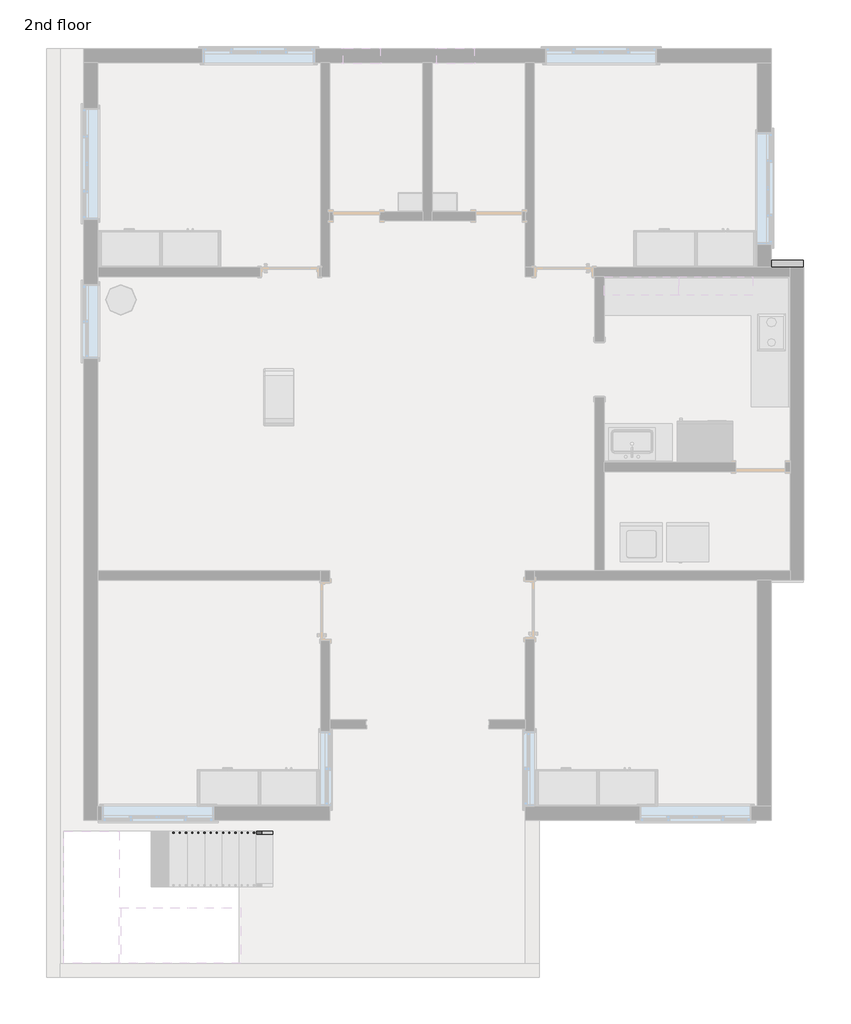
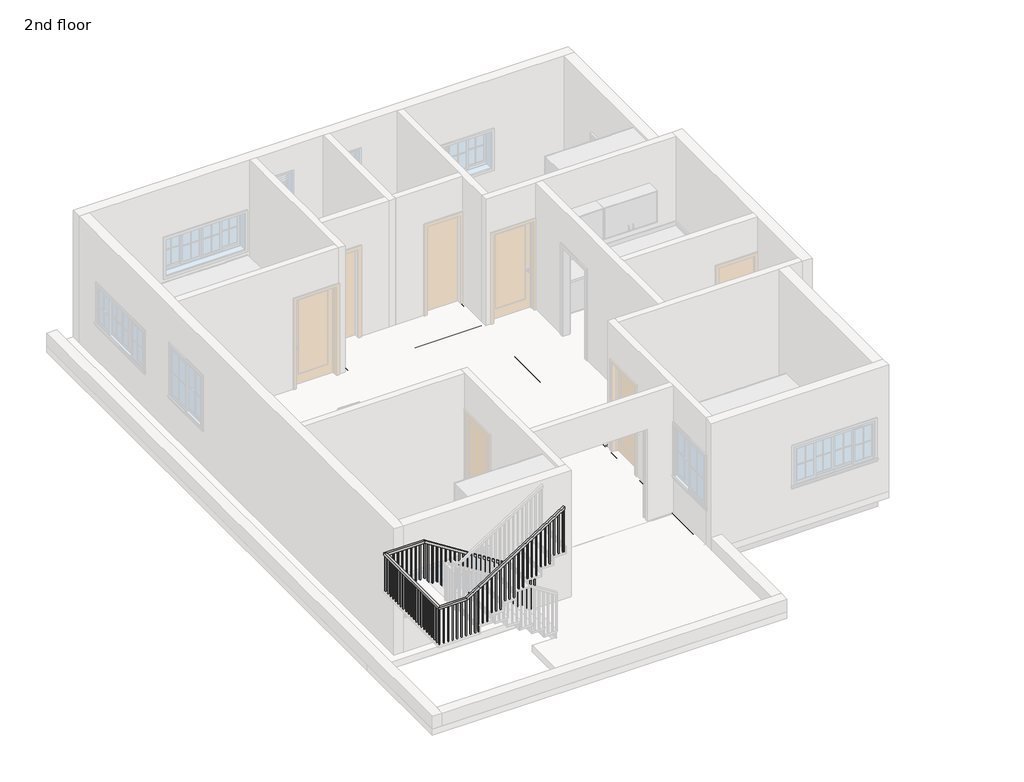
# One storey, part 2 of 4: 6 beams, 1 railing.
"""IFC4 building model written with IfcOpenShell, lengths in millimetres."""

from ifc_helpers import new_model, si_unit, frame, origin, place, context, project, spatial, polyline, outline, extrude, faceted_brep, element, save

model = new_model("IFC4")

# Units and contexts
model_context = context("Model", 3, world=origin())
ifc_project = project(units=[si_unit("LENGTHUNIT", "METRE", prefix="MILLI")], contexts=[model_context])

# Site, building, storey
site = spatial("IfcSite", under=ifc_project)
building = spatial("IfcBuilding", under=site)
storey = spatial("IfcBuildingStorey", under=building, Name="2nd floor", Elevation=7010.4)

# Beams
placement = place(None, origin())
element("IfcBeam", 1, ObjectType="Concrete-Rectangular Beam", at=placement, inside=storey, context=model_context, shape_type="Brep", body=[
    faceted_brep([(-12413.6124084, 10142.6961804, 7010.4), (-12413.6124084, 9914.0961804, 7010.4), (-8794.1124084, 9914.0961804, 7010.4), (-8565.5124084, 9914.0961804, 7010.4), (-7117.7124084, 9914.0961804, 7010.4), (-6889.1124084, 9914.0961804, 7010.4), (-5441.3124084, 9914.0961804, 7010.4), (-5212.7124084, 9914.0961804, 7010.4), (-1593.2124084, 9914.0961804, 7010.4), (-1593.2124084, 10142.6961804, 7010.4), (-5174.6124084, 10142.6961804, 7010.4), (-5174.6124084, 9952.1961804, 7010.4), (-5479.4124084, 9952.1961804, 7010.4), (-5479.4124084, 10142.6961804, 7010.4), (-8451.2124084, 10142.6961804, 7010.4), (-8451.2124084, 9952.1961804, 7010.4), (-8756.0124084, 9952.1961804, 7010.4), (-8756.0124084, 10142.6961804, 7010.4), (-12413.6124084, 9914.0961804, 6705.6), (-8794.1124084, 9914.0961804, 6705.6), (-8565.5124084, 9914.0961804, 6705.6), (-7117.7124084, 9914.0961804, 6705.6), (-6889.1124084, 9914.0961804, 6705.6), (-5441.3124084, 9914.0961804, 6705.6), (-5212.7124084, 9914.0961804, 6705.6), (-1593.2124084, 9914.0961804, 6705.6), (-12413.6124084, 10142.6961804, 6705.6), (-8756.0124084, 10142.6961804, 6705.6), (-8756.0124084, 9952.1961804, 6705.6), (-8451.2124084, 9952.1961804, 6705.6), (-8451.2124084, 10142.6961804, 6705.6), (-5479.4124084, 10142.6961804, 6705.6), (-5479.4124084, 9952.1961804, 6705.6), (-5174.6124084, 9952.1961804, 6705.6), (-5174.6124084, 10142.6961804, 6705.6), (-1593.2124084, 10142.6961804, 6705.6)], [[[0, 1, 2, 3, 4, 5, 6, 7, 8, 9, 10, 11, 12, 13, 14, 15, 16, 17]], [[1, 18, 19, 20, 21, 22, 23, 24, 25, 8, 7, 6, 5, 4, 3, 2]], [[18, 26, 27, 28, 29, 30, 31, 32, 33, 34, 35, 25, 24, 23, 22, 21, 20, 19]], [[26, 0, 17, 27]], [[1, 0, 26, 18]], [[9, 8, 25, 35]], [[29, 15, 14, 30]], [[15, 29, 28, 16]], [[16, 28, 27, 17]], [[9, 35, 34, 10]], [[33, 11, 10, 34]], [[11, 33, 32, 12]], [[12, 32, 31, 13]], [[30, 14, 13, 31]]]),
])
element("IfcBeam", 2, ObjectType="Concrete-Rectangular Beam", at=placement, inside=storey, context=model_context, shape_type="SweptSolid", body=[
    extrude(outline(polyline([(-1593.2124084, 9875.9961804), (-1364.6124084, 9875.9961804), (-1364.6124084, 6751.7961804), (-1593.2124084, 6751.7961804), (-1593.2124084, 9875.9961804)])), frame((0.0, 0.0, 6705.6), z_axis=(0.0, 0.0, 1.0), x_axis=(1.0, 0.0, 0.0)), (0.0, 0.0, 1.0), 304.8),
])
element("IfcBeam", 3, ObjectType="Concrete-Rectangular Beam", at=placement, inside=storey, context=model_context, shape_type="Brep", body=[
    faceted_brep([(-843.9124084, 6713.6961804, 7010.4), (-843.9124084, 6485.0961804, 7010.4), (-843.9124084, 6485.0961804, 6705.6), (-843.9124084, 6713.6961804, 6705.6), (-1364.6124084, 6713.6961804, 7010.4), (-1364.6124084, 6485.0961804, 7010.4), (-1364.6124084, 6485.0961804, 6705.6), (-1364.6124084, 6713.6961804, 6705.6)], [[[0, 1, 2, 3]], [[1, 0, 4, 5]], [[2, 1, 5, 6]], [[3, 2, 6, 7]], [[0, 3, 7, 4]], [[5, 4, 7, 6]]]),
    faceted_brep([(-12413.6124084, 6485.0961804, 7010.4), (-12413.6124084, 6713.6961804, 7010.4), (-12413.6124084, 6713.6961804, 6705.6), (-12413.6124084, 6485.0961804, 6705.6), (-8756.0124084, 6713.6961804, 7010.4), (-8756.0124084, 6485.0961804, 7010.4), (-8756.0124084, 6485.0961804, 6705.6), (-8756.0124084, 6713.6961804, 6705.6), (-8794.1124084, 6485.0961804, 7010.4), (-8794.1124084, 6713.6961804, 7010.4), (-8794.1124084, 6485.0961804, 6705.6), (-8794.1124084, 6713.6961804, 6705.6)], [[[0, 1, 2, 3]], [[4, 5, 6, 7]], [[1, 0, 8, 5, 4, 9]], [[0, 3, 10, 6, 5, 8]], [[3, 2, 11, 7, 6, 10]], [[2, 1, 9, 4, 7, 11]]]),
    faceted_brep([(-1593.2124084, 6713.6961804, 7010.4), (-1593.2124084, 6485.0961804, 7010.4), (-1593.2124084, 6485.0961804, 6705.6), (-1593.2124084, 6713.6961804, 6705.6), (-5212.7124084, 6713.6961804, 7010.4), (-5250.8124084, 6713.6961804, 7010.4), (-5250.8124084, 6485.0961804, 7010.4), (-5212.7124084, 6485.0961804, 7010.4), (-5250.8124084, 6485.0961804, 6705.6), (-5212.7124084, 6485.0961804, 6705.6), (-5250.8124084, 6713.6961804, 6705.6), (-5212.7124084, 6713.6961804, 6705.6)], [[[0, 1, 2, 3]], [[1, 0, 4, 5, 6, 7]], [[2, 1, 7, 6, 8, 9]], [[3, 2, 9, 8, 10, 11]], [[0, 3, 11, 10, 5, 4]], [[6, 5, 10, 8]]]),
    faceted_brep([(-8527.4124084, 6485.0961804, 7010.4), (-8527.4124084, 6713.6961804, 7010.4), (-8527.4124084, 6713.6961804, 6705.6), (-8527.4124084, 6485.0961804, 6705.6), (-5479.4124084, 6713.6961804, 7010.4), (-5479.4124084, 6485.0961804, 7010.4), (-5479.4124084, 6485.0961804, 6705.6), (-5479.4124084, 6713.6961804, 6705.6)], [[[0, 1, 2, 3]], [[4, 5, 6, 7]], [[1, 0, 5, 4]], [[0, 3, 6, 5]], [[3, 2, 7, 6]], [[2, 1, 4, 7]]]),
])
element("IfcBeam", 4, ObjectType="Concrete-Rectangular Beam", at=placement, inside=storey, context=model_context, shape_type="Brep", body=[
    faceted_brep([(-5212.7124084, 9914.0961804, 7010.4), (-5441.3124084, 9914.0961804, 7010.4), (-5441.3124084, 7551.8961804, 7010.4), (-5441.3124084, 7323.2961804, 7010.4), (-5441.3124084, 6751.7961804, 7010.4), (-5250.8124084, 6751.7961804, 7010.4), (-5250.8124084, 6713.6961804, 7010.4), (-5212.7124084, 6713.6961804, 7010.4), (-5212.7124084, 9914.0961804, 6705.6), (-5212.7124084, 6713.6961804, 6705.6), (-5441.3124084, 9914.0961804, 6705.6), (-5250.8124084, 6713.6961804, 6705.6), (-5250.8124084, 6751.7961804, 6705.6), (-5441.3124084, 6751.7961804, 6705.6), (-5441.3124084, 7323.2961804, 6705.6), (-5441.3124084, 7551.8961804, 6705.6)], [[[0, 1, 2, 3, 4, 5, 6, 7]], [[8, 0, 7, 9]], [[10, 8, 9, 11, 12, 13, 14, 15]], [[1, 10, 15, 14, 13, 4, 3, 2]], [[1, 0, 8, 10]], [[9, 7, 6, 11]], [[12, 5, 4, 13]], [[5, 12, 11, 6]]]),
    faceted_brep([(-5212.7124084, -2201.7038196, 7010.4), (-5441.3124084, -2201.7038196, 7010.4), (-5441.3124084, -2201.7038196, 6705.6), (-5212.7124084, -2201.7038196, 6705.6), (-5441.3124084, 1430.4961804, 6705.6), (-5441.3124084, 1430.4961804, 7010.4), (-5212.7124084, 1430.4961804, 7010.4), (-5212.7124084, 1430.4961804, 6705.6), (-5441.3124084, -779.3038196, 6705.6), (-5441.3124084, -1007.9038196, 6705.6), (-5441.3124084, -1007.9038196, 7010.4), (-5441.3124084, -779.3038196, 7010.4)], [[[0, 1, 2, 3]], [[4, 5, 6, 7]], [[5, 4, 8, 9, 2, 1, 10, 11]], [[1, 0, 6, 5, 11, 10]], [[0, 3, 7, 6]], [[3, 2, 9, 8, 4, 7]]]),
    faceted_brep([(-5212.7124084, 6485.0961804, 7010.4), (-5212.7124084, 6485.0961804, 6705.6), (-5250.8124084, 6485.0961804, 6705.6), (-5250.8124084, 6485.0961804, 7010.4), (-5250.8124084, 6446.9961804, 7010.4), (-5441.3124084, 6446.9961804, 7010.4), (-5441.3124084, 1659.0961804, 7010.4), (-5403.2124084, 1659.0961804, 7010.4), (-5403.2124084, 1697.1961804, 7010.4), (-5212.7124084, 1697.1961804, 7010.4), (-5212.7124084, 1697.1961804, 6705.6), (-5403.2124084, 1697.1961804, 6705.6), (-5403.2124084, 1659.0961804, 6705.6), (-5441.3124084, 1659.0961804, 6705.6), (-5441.3124084, 6446.9961804, 6705.6), (-5250.8124084, 6446.9961804, 6705.6)], [[[0, 1, 2, 3]], [[0, 3, 4, 5, 6, 7, 8, 9]], [[1, 0, 9, 10]], [[2, 1, 10, 11, 12, 13, 14, 15]], [[6, 13, 12, 7]], [[13, 6, 5, 14]], [[15, 4, 3, 2]], [[4, 15, 14, 5]], [[8, 11, 10, 9]], [[11, 8, 7, 12]]]),
])
element("IfcBeam", 5, ObjectType="Concrete-Rectangular Beam", at=placement, inside=storey, context=model_context, shape_type="SweptSolid", body=[
    extrude(outline(polyline([(-7117.7124084, 9914.0961804), (-6889.1124084, 9914.0961804), (-6889.1124084, 7551.8961804), (-7117.7124084, 7551.8961804), (-7117.7124084, 9914.0961804)])), frame((0.0, 0.0, 6705.6), z_axis=(0.0, 0.0, 1.0), x_axis=(1.0, 0.0, 0.0)), (0.0, 0.0, 1.0), 304.8),
])
element("IfcBeam", 6, ObjectType="Concrete-Rectangular Beam", at=placement, inside=storey, context=model_context, shape_type="Brep", body=[
    faceted_brep([(-5441.3124084, 7323.2961804, 7010.4), (-5441.3124084, 7551.8961804, 7010.4), (-6889.1124084, 7551.8961804, 7010.4), (-7117.7124084, 7551.8961804, 7010.4), (-8565.5124084, 7551.8961804, 7010.4), (-8565.5124084, 7323.2961804, 7010.4), (-5441.3124084, 7323.2961804, 6705.6), (-8565.5124084, 7323.2961804, 6705.6), (-5441.3124084, 7551.8961804, 6705.6), (-8565.5124084, 7551.8961804, 6705.6), (-7117.7124084, 7551.8961804, 6705.6), (-6889.1124084, 7551.8961804, 6705.6)], [[[0, 1, 2, 3, 4, 5]], [[6, 0, 5, 7]], [[8, 6, 7, 9, 10, 11]], [[1, 8, 11, 10, 9, 4, 3, 2]], [[1, 0, 6, 8]], [[5, 4, 9, 7]]]),
])

# Railing
element("IfcRailing", 7, ObjectType="Handrail - Rectangular", at=placement, inside=storey, context=model_context, shape_type="SolidModel", body=[
    faceted_brep([(-9543.8120641, -2698.7669819, 8102.6), (-9543.8120641, -2698.7669819, 8042.386276), (-9543.8120641, -2647.9669819, 8042.386276), (-9543.8120641, -2647.9669819, 8102.6), (-12058.4120641, -2698.7669819, 9702.8), (-12073.205059, -2698.7669819, 9652.0), (-12073.205059, -2647.9669819, 9652.0), (-12058.4120641, -2647.9669819, 9702.8), (-12922.0120641, -2698.7669819, 9702.8), (-12922.0120641, -2698.7669819, 9652.0), (-12972.8120641, -2647.9669819, 9652.0), (-12972.8120641, -2647.9669819, 9702.8), (-12922.0120641, -4767.1038196, 9702.8), (-12922.0120641, -4767.1038196, 9652.0), (-12972.8120641, -4817.9038196, 9652.0), (-12972.8120641, -4817.9038196, 9702.8), (-12337.8120641, -4767.1038196, 9702.8), (-12323.0190691, -4767.1038196, 9652.0), (-12323.0190691, -4817.9038196, 9652.0), (-12337.8120641, -4817.9038196, 9702.8), (-12058.4120641, -4767.1038196, 9880.6), (-12031.138789, -4767.1038196, 9837.7419964), (-12031.138789, -4817.9038196, 9837.7419964), (-12058.4120641, -4817.9038196, 9880.6), (-10102.6120641, -4767.1038196, 11125.2), (-10102.6120641, -4817.9038196, 11125.2), (-10102.6120641, -4817.9038196, 11064.986276), (-10102.6120641, -4767.1038196, 11064.986276)], [[[0, 1, 2, 3]], [[1, 0, 4, 5]], [[2, 1, 5, 6]], [[3, 2, 6, 7]], [[0, 3, 7, 4]], [[5, 4, 8, 9]], [[6, 5, 9, 10]], [[7, 6, 10, 11]], [[4, 7, 11, 8]], [[9, 8, 12, 13]], [[10, 9, 13, 14]], [[11, 10, 14, 15]], [[8, 11, 15, 12]], [[13, 12, 16, 17]], [[14, 13, 17, 18]], [[15, 14, 18, 19]], [[12, 15, 19, 16]], [[17, 16, 20, 21]], [[18, 17, 21, 22]], [[19, 18, 22, 23]], [[16, 19, 23, 20]], [[24, 25, 26, 27]], [[21, 20, 24, 27]], [[22, 21, 27, 26]], [[23, 22, 26, 25]], [[20, 23, 25, 24]]]),
    extrude(outline(polyline([(11054.8840032, -10118.4870641), (11042.761276, -10137.5370641), (10033.0, -10137.5370641), (10033.0, -10118.4870641), (11054.8840032, -10118.4870641)])), frame((0.0, -4802.0288196, 0.0), z_axis=(0.0, 1.0, 0.0), x_axis=(0.0, 0.0, 1.0)), (0.0, 0.0, 1.0), 19.05),
    extrude(outline(polyline([(10990.2294578, -10220.0870641), (10978.1067305, -10239.1370641), (10033.0, -10239.1370641), (10033.0, -10220.0870641), (10990.2294578, -10220.0870641)])), frame((0.0, -4802.0288196, 0.0), z_axis=(0.0, 1.0, 0.0), x_axis=(0.0, 0.0, 1.0)), (0.0, 0.0, 1.0), 19.05),
    extrude(outline(polyline([(10925.5749123, -10321.6870641), (10913.4521851, -10340.7370641), (10033.0, -10340.7370641), (10033.0, -10321.6870641), (10925.5749123, -10321.6870641)])), frame((0.0, -4802.0288196, 0.0), z_axis=(0.0, 1.0, 0.0), x_axis=(0.0, 0.0, 1.0)), (0.0, 0.0, 1.0), 19.05),
    extrude(outline(polyline([(10860.9203669, -10423.2870641), (10848.7976396, -10442.3370641), (9855.2, -10442.3370641), (9855.2, -10423.2870641), (10860.9203669, -10423.2870641)])), frame((0.0, -4802.0288196, 0.0), z_axis=(0.0, 1.0, 0.0), x_axis=(0.0, 0.0, 1.0)), (0.0, 0.0, 1.0), 19.05),
    extrude(outline(polyline([(10796.2658214, -10524.8870641), (10784.1430941, -10543.9370641), (9855.2, -10543.9370641), (9855.2, -10524.8870641), (10796.2658214, -10524.8870641)])), frame((0.0, -4802.0288196, 0.0), z_axis=(0.0, 1.0, 0.0), x_axis=(0.0, 0.0, 1.0)), (0.0, 0.0, 1.0), 19.05),
    extrude(outline(polyline([(10731.611276, -10626.4870641), (10719.4885487, -10645.5370641), (9855.2, -10645.5370641), (9855.2, -10626.4870641), (10731.611276, -10626.4870641)])), frame((0.0, -4802.0288196, 0.0), z_axis=(0.0, 1.0, 0.0), x_axis=(0.0, 0.0, 1.0)), (0.0, 0.0, 1.0), 19.05),
    extrude(outline(polyline([(10666.9567305, -10728.0870641), (10654.8340032, -10747.1370641), (9677.4, -10747.1370641), (9677.4, -10728.0870641), (10666.9567305, -10728.0870641)])), frame((0.0, -4802.0288196, 0.0), z_axis=(0.0, 1.0, 0.0), x_axis=(0.0, 0.0, 1.0)), (0.0, 0.0, 1.0), 19.05),
    extrude(outline(polyline([(10602.3021851, -10829.6870641), (10590.1794578, -10848.7370641), (9677.4, -10848.7370641), (9677.4, -10829.6870641), (10602.3021851, -10829.6870641)])), frame((0.0, -4802.0288196, 0.0), z_axis=(0.0, 1.0, 0.0), x_axis=(0.0, 0.0, 1.0)), (0.0, 0.0, 1.0), 19.05),
    extrude(outline(polyline([(10537.6476396, -10931.2870641), (10525.5249123, -10950.3370641), (9677.4, -10950.3370641), (9677.4, -10931.2870641), (10537.6476396, -10931.2870641)])), frame((0.0, -4802.0288196, 0.0), z_axis=(0.0, 1.0, 0.0), x_axis=(0.0, 0.0, 1.0)), (0.0, 0.0, 1.0), 19.05),
    extrude(outline(polyline([(10472.9930941, -11032.8870641), (10460.8703669, -11051.9370641), (9499.6, -11051.9370641), (9499.6, -11032.8870641), (10472.9930941, -11032.8870641)])), frame((0.0, -4802.0288196, 0.0), z_axis=(0.0, 1.0, 0.0), x_axis=(0.0, 0.0, 1.0)), (0.0, 0.0, 1.0), 19.05),
    extrude(outline(polyline([(10408.3385487, -11134.4870641), (10396.2158214, -11153.5370641), (9499.6, -11153.5370641), (9499.6, -11134.4870641), (10408.3385487, -11134.4870641)])), frame((0.0, -4802.0288196, 0.0), z_axis=(0.0, 1.0, 0.0), x_axis=(0.0, 0.0, 1.0)), (0.0, 0.0, 1.0), 19.05),
    extrude(outline(polyline([(10343.6840032, -11236.0870641), (10331.561276, -11255.1370641), (9321.8, -11255.1370641), (9321.8, -11236.0870641), (10343.6840032, -11236.0870641)])), frame((0.0, -4802.0288196, 0.0), z_axis=(0.0, 1.0, 0.0), x_axis=(0.0, 0.0, 1.0)), (0.0, 0.0, 1.0), 19.05),
    extrude(outline(polyline([(10279.0294578, -11337.6870641), (10266.9067305, -11356.7370641), (9321.8, -11356.7370641), (9321.8, -11337.6870641), (10279.0294578, -11337.6870641)])), frame((0.0, -4802.0288196, 0.0), z_axis=(0.0, 1.0, 0.0), x_axis=(0.0, 0.0, 1.0)), (0.0, 0.0, 1.0), 19.05),
    extrude(outline(polyline([(10214.3749123, -11439.2870641), (10202.2521851, -11458.3370641), (9321.8, -11458.3370641), (9321.8, -11439.2870641), (10214.3749123, -11439.2870641)])), frame((0.0, -4802.0288196, 0.0), z_axis=(0.0, 1.0, 0.0), x_axis=(0.0, 0.0, 1.0)), (0.0, 0.0, 1.0), 19.05),
    extrude(outline(polyline([(10149.7203669, -11540.8870641), (10137.5976396, -11559.9370641), (9144.0, -11559.9370641), (9144.0, -11540.8870641), (10149.7203669, -11540.8870641)])), frame((0.0, -4802.0288196, 0.0), z_axis=(0.0, 1.0, 0.0), x_axis=(0.0, 0.0, 1.0)), (0.0, 0.0, 1.0), 19.05),
    extrude(outline(polyline([(10085.0658214, -11642.4870641), (10072.9430941, -11661.5370641), (9144.0, -11661.5370641), (9144.0, -11642.4870641), (10085.0658214, -11642.4870641)])), frame((0.0, -4802.0288196, 0.0), z_axis=(0.0, 1.0, 0.0), x_axis=(0.0, 0.0, 1.0)), (0.0, 0.0, 1.0), 19.05),
    extrude(outline(polyline([(10020.411276, -11744.0870641), (10008.2885487, -11763.1370641), (9144.0, -11763.1370641), (9144.0, -11744.0870641), (10020.411276, -11744.0870641)])), frame((0.0, -4802.0288196, 0.0), z_axis=(0.0, 1.0, 0.0), x_axis=(0.0, 0.0, 1.0)), (0.0, 0.0, 1.0), 19.05),
    extrude(outline(polyline([(9955.7567305, -11845.6870641), (9943.6340032, -11864.7370641), (8966.2, -11864.7370641), (8966.2, -11845.6870641), (9955.7567305, -11845.6870641)])), frame((0.0, -4802.0288196, 0.0), z_axis=(0.0, 1.0, 0.0), x_axis=(0.0, 0.0, 1.0)), (0.0, 0.0, 1.0), 19.05),
    extrude(outline(polyline([(9891.1021851, -11947.2870641), (9878.9794578, -11966.3370641), (8966.2, -11966.3370641), (8966.2, -11947.2870641), (9891.1021851, -11947.2870641)])), frame((0.0, -4802.0288196, 0.0), z_axis=(0.0, 1.0, 0.0), x_axis=(0.0, 0.0, 1.0)), (0.0, 0.0, 1.0), 19.05),
    extrude(outline(polyline([(9777.9567305, -12125.0870641), (9765.8340032, -12144.1370641), (8788.4, -12144.1370641), (8788.4, -12125.0870641), (9777.9567305, -12125.0870641)])), frame((0.0, -4802.0288196, 0.0), z_axis=(0.0, 1.0, 0.0), x_axis=(0.0, 0.0, 1.0)), (0.0, 0.0, 1.0), 19.05),
    extrude(outline(polyline([(9713.3021851, -12226.6870641), (9701.1794578, -12245.7370641), (8788.4, -12245.7370641), (8788.4, -12226.6870641), (9713.3021851, -12226.6870641)])), frame((0.0, -4802.0288196, 0.0), z_axis=(0.0, 1.0, 0.0), x_axis=(0.0, 0.0, 1.0)), (0.0, 0.0, 1.0), 19.05),
    extrude(outline(polyline([(-12347.3370641, -4802.0288196), (-12347.3370641, -4782.9788196), (-12328.2870641, -4782.9788196), (-12328.2870641, -4802.0288196), (-12347.3370641, -4802.0288196)])), frame((0.0, 0.0, 8788.4), z_axis=(0.0, 0.0, 1.0), x_axis=(1.0, 0.0, 0.0)), (0.0, 0.0, 1.0), 863.6),
    extrude(outline(polyline([(-12448.9370641, -4802.0288196), (-12448.9370641, -4782.9788196), (-12429.8870641, -4782.9788196), (-12429.8870641, -4802.0288196), (-12448.9370641, -4802.0288196)])), frame((0.0, 0.0, 8788.4), z_axis=(0.0, 0.0, 1.0), x_axis=(1.0, 0.0, 0.0)), (0.0, 0.0, 1.0), 863.6),
    extrude(outline(polyline([(-12550.5370641, -4802.0288196), (-12550.5370641, -4782.9788196), (-12531.4870641, -4782.9788196), (-12531.4870641, -4802.0288196), (-12550.5370641, -4802.0288196)])), frame((0.0, 0.0, 8788.4), z_axis=(0.0, 0.0, 1.0), x_axis=(1.0, 0.0, 0.0)), (0.0, 0.0, 1.0), 863.6),
    extrude(outline(polyline([(-12652.1370641, -4802.0288196), (-12652.1370641, -4782.9788196), (-12633.0870641, -4782.9788196), (-12633.0870641, -4802.0288196), (-12652.1370641, -4802.0288196)])), frame((0.0, 0.0, 8788.4), z_axis=(0.0, 0.0, 1.0), x_axis=(1.0, 0.0, 0.0)), (0.0, 0.0, 1.0), 863.6),
    extrude(outline(polyline([(-12753.7370641, -4802.0288196), (-12753.7370641, -4782.9788196), (-12734.6870641, -4782.9788196), (-12734.6870641, -4802.0288196), (-12753.7370641, -4802.0288196)])), frame((0.0, 0.0, 8788.4), z_axis=(0.0, 0.0, 1.0), x_axis=(1.0, 0.0, 0.0)), (0.0, 0.0, 1.0), 863.6),
    extrude(outline(polyline([(-12855.3370641, -4802.0288196), (-12855.3370641, -4782.9788196), (-12836.2870641, -4782.9788196), (-12836.2870641, -4802.0288196), (-12855.3370641, -4802.0288196)])), frame((0.0, 0.0, 8788.4), z_axis=(0.0, 0.0, 1.0), x_axis=(1.0, 0.0, 0.0)), (0.0, 0.0, 1.0), 863.6),
    extrude(outline(polyline([(-12956.9370641, -4695.8419819), (-12937.8870641, -4695.8419819), (-12937.8870641, -4714.8919819), (-12956.9370641, -4714.8919819), (-12956.9370641, -4695.8419819)])), frame((0.0, 0.0, 8788.4), z_axis=(0.0, 0.0, 1.0), x_axis=(1.0, 0.0, 0.0)), (0.0, 0.0, 1.0), 863.6),
    extrude(outline(polyline([(-12956.9370641, -4594.2419819), (-12937.8870641, -4594.2419819), (-12937.8870641, -4613.2919819), (-12956.9370641, -4613.2919819), (-12956.9370641, -4594.2419819)])), frame((0.0, 0.0, 8788.4), z_axis=(0.0, 0.0, 1.0), x_axis=(1.0, 0.0, 0.0)), (0.0, 0.0, 1.0), 863.6),
    extrude(outline(polyline([(-12956.9370641, -4492.6419819), (-12937.8870641, -4492.6419819), (-12937.8870641, -4511.6919819), (-12956.9370641, -4511.6919819), (-12956.9370641, -4492.6419819)])), frame((0.0, 0.0, 8788.4), z_axis=(0.0, 0.0, 1.0), x_axis=(1.0, 0.0, 0.0)), (0.0, 0.0, 1.0), 863.6),
    extrude(outline(polyline([(-12956.9370641, -4391.0419819), (-12937.8870641, -4391.0419819), (-12937.8870641, -4410.0919819), (-12956.9370641, -4410.0919819), (-12956.9370641, -4391.0419819)])), frame((0.0, 0.0, 8788.4), z_axis=(0.0, 0.0, 1.0), x_axis=(1.0, 0.0, 0.0)), (0.0, 0.0, 1.0), 863.6),
    extrude(outline(polyline([(-12956.9370641, -4289.4419819), (-12937.8870641, -4289.4419819), (-12937.8870641, -4308.4919819), (-12956.9370641, -4308.4919819), (-12956.9370641, -4289.4419819)])), frame((0.0, 0.0, 8788.4), z_axis=(0.0, 0.0, 1.0), x_axis=(1.0, 0.0, 0.0)), (0.0, 0.0, 1.0), 863.6),
    extrude(outline(polyline([(-12956.9370641, -4187.8419819), (-12937.8870641, -4187.8419819), (-12937.8870641, -4206.8919819), (-12956.9370641, -4206.8919819), (-12956.9370641, -4187.8419819)])), frame((0.0, 0.0, 8788.4), z_axis=(0.0, 0.0, 1.0), x_axis=(1.0, 0.0, 0.0)), (0.0, 0.0, 1.0), 863.6),
    extrude(outline(polyline([(-12956.9370641, -4086.2419819), (-12937.8870641, -4086.2419819), (-12937.8870641, -4105.2919819), (-12956.9370641, -4105.2919819), (-12956.9370641, -4086.2419819)])), frame((0.0, 0.0, 8788.4), z_axis=(0.0, 0.0, 1.0), x_axis=(1.0, 0.0, 0.0)), (0.0, 0.0, 1.0), 863.6),
    extrude(outline(polyline([(-12956.9370641, -3984.6419819), (-12937.8870641, -3984.6419819), (-12937.8870641, -4003.6919819), (-12956.9370641, -4003.6919819), (-12956.9370641, -3984.6419819)])), frame((0.0, 0.0, 8788.4), z_axis=(0.0, 0.0, 1.0), x_axis=(1.0, 0.0, 0.0)), (0.0, 0.0, 1.0), 863.6),
    extrude(outline(polyline([(-12956.9370641, -3883.0419819), (-12937.8870641, -3883.0419819), (-12937.8870641, -3902.0919819), (-12956.9370641, -3902.0919819), (-12956.9370641, -3883.0419819)])), frame((0.0, 0.0, 8788.4), z_axis=(0.0, 0.0, 1.0), x_axis=(1.0, 0.0, 0.0)), (0.0, 0.0, 1.0), 863.6),
    extrude(outline(polyline([(-12956.9370641, -3781.4419819), (-12937.8870641, -3781.4419819), (-12937.8870641, -3800.4919819), (-12956.9370641, -3800.4919819), (-12956.9370641, -3781.4419819)])), frame((0.0, 0.0, 8788.4), z_axis=(0.0, 0.0, 1.0), x_axis=(1.0, 0.0, 0.0)), (0.0, 0.0, 1.0), 863.6),
    extrude(outline(polyline([(-12956.9370641, -3679.8419819), (-12937.8870641, -3679.8419819), (-12937.8870641, -3698.8919819), (-12956.9370641, -3698.8919819), (-12956.9370641, -3679.8419819)])), frame((0.0, 0.0, 8788.4), z_axis=(0.0, 0.0, 1.0), x_axis=(1.0, 0.0, 0.0)), (0.0, 0.0, 1.0), 863.6),
    extrude(outline(polyline([(-12956.9370641, -3578.2419819), (-12937.8870641, -3578.2419819), (-12937.8870641, -3597.2919819), (-12956.9370641, -3597.2919819), (-12956.9370641, -3578.2419819)])), frame((0.0, 0.0, 8788.4), z_axis=(0.0, 0.0, 1.0), x_axis=(1.0, 0.0, 0.0)), (0.0, 0.0, 1.0), 863.6),
    extrude(outline(polyline([(-12956.9370641, -3476.6419819), (-12937.8870641, -3476.6419819), (-12937.8870641, -3495.6919819), (-12956.9370641, -3495.6919819), (-12956.9370641, -3476.6419819)])), frame((0.0, 0.0, 8788.4), z_axis=(0.0, 0.0, 1.0), x_axis=(1.0, 0.0, 0.0)), (0.0, 0.0, 1.0), 863.6),
    extrude(outline(polyline([(-12956.9370641, -3375.0419819), (-12937.8870641, -3375.0419819), (-12937.8870641, -3394.0919819), (-12956.9370641, -3394.0919819), (-12956.9370641, -3375.0419819)])), frame((0.0, 0.0, 8788.4), z_axis=(0.0, 0.0, 1.0), x_axis=(1.0, 0.0, 0.0)), (0.0, 0.0, 1.0), 863.6),
    extrude(outline(polyline([(-12956.9370641, -3273.4419819), (-12937.8870641, -3273.4419819), (-12937.8870641, -3292.4919819), (-12956.9370641, -3292.4919819), (-12956.9370641, -3273.4419819)])), frame((0.0, 0.0, 8788.4), z_axis=(0.0, 0.0, 1.0), x_axis=(1.0, 0.0, 0.0)), (0.0, 0.0, 1.0), 863.6),
    extrude(outline(polyline([(-12956.9370641, -3171.8419819), (-12937.8870641, -3171.8419819), (-12937.8870641, -3190.8919819), (-12956.9370641, -3190.8919819), (-12956.9370641, -3171.8419819)])), frame((0.0, 0.0, 8788.4), z_axis=(0.0, 0.0, 1.0), x_axis=(1.0, 0.0, 0.0)), (0.0, 0.0, 1.0), 863.6),
    extrude(outline(polyline([(-12956.9370641, -3070.2419819), (-12937.8870641, -3070.2419819), (-12937.8870641, -3089.2919819), (-12956.9370641, -3089.2919819), (-12956.9370641, -3070.2419819)])), frame((0.0, 0.0, 8788.4), z_axis=(0.0, 0.0, 1.0), x_axis=(1.0, 0.0, 0.0)), (0.0, 0.0, 1.0), 863.6),
    extrude(outline(polyline([(-12956.9370641, -2968.6419819), (-12937.8870641, -2968.6419819), (-12937.8870641, -2987.6919819), (-12956.9370641, -2987.6919819), (-12956.9370641, -2968.6419819)])), frame((0.0, 0.0, 8788.4), z_axis=(0.0, 0.0, 1.0), x_axis=(1.0, 0.0, 0.0)), (0.0, 0.0, 1.0), 863.6),
    extrude(outline(polyline([(-12956.9370641, -2867.0419819), (-12937.8870641, -2867.0419819), (-12937.8870641, -2886.0919819), (-12956.9370641, -2886.0919819), (-12956.9370641, -2867.0419819)])), frame((0.0, 0.0, 8788.4), z_axis=(0.0, 0.0, 1.0), x_axis=(1.0, 0.0, 0.0)), (0.0, 0.0, 1.0), 863.6),
    extrude(outline(polyline([(-12956.9370641, -2765.4419819), (-12937.8870641, -2765.4419819), (-12937.8870641, -2784.4919819), (-12956.9370641, -2784.4919819), (-12956.9370641, -2765.4419819)])), frame((0.0, 0.0, 8788.4), z_axis=(0.0, 0.0, 1.0), x_axis=(1.0, 0.0, 0.0)), (0.0, 0.0, 1.0), 863.6),
    extrude(outline(polyline([(-12861.6870641, -2663.8419819), (-12861.6870641, -2682.8919819), (-12880.7370641, -2682.8919819), (-12880.7370641, -2663.8419819), (-12861.6870641, -2663.8419819)])), frame((0.0, 0.0, 8788.4), z_axis=(0.0, 0.0, 1.0), x_axis=(1.0, 0.0, 0.0)), (0.0, 0.0, 1.0), 863.6),
    extrude(outline(polyline([(-12760.0870641, -2663.8419819), (-12760.0870641, -2682.8919819), (-12779.1370641, -2682.8919819), (-12779.1370641, -2663.8419819), (-12760.0870641, -2663.8419819)])), frame((0.0, 0.0, 8788.4), z_axis=(0.0, 0.0, 1.0), x_axis=(1.0, 0.0, 0.0)), (0.0, 0.0, 1.0), 863.6),
    extrude(outline(polyline([(-12658.4870641, -2663.8419819), (-12658.4870641, -2682.8919819), (-12677.5370641, -2682.8919819), (-12677.5370641, -2663.8419819), (-12658.4870641, -2663.8419819)])), frame((0.0, 0.0, 8788.4), z_axis=(0.0, 0.0, 1.0), x_axis=(1.0, 0.0, 0.0)), (0.0, 0.0, 1.0), 863.6),
    extrude(outline(polyline([(-12556.8870641, -2663.8419819), (-12556.8870641, -2682.8919819), (-12575.9370641, -2682.8919819), (-12575.9370641, -2663.8419819), (-12556.8870641, -2663.8419819)])), frame((0.0, 0.0, 8788.4), z_axis=(0.0, 0.0, 1.0), x_axis=(1.0, 0.0, 0.0)), (0.0, 0.0, 1.0), 863.6),
    extrude(outline(polyline([(-12455.2870641, -2663.8419819), (-12455.2870641, -2682.8919819), (-12474.3370641, -2682.8919819), (-12474.3370641, -2663.8419819), (-12455.2870641, -2663.8419819)])), frame((0.0, 0.0, 8788.4), z_axis=(0.0, 0.0, 1.0), x_axis=(1.0, 0.0, 0.0)), (0.0, 0.0, 1.0), 863.6),
    extrude(outline(polyline([(-12353.6870641, -2663.8419819), (-12353.6870641, -2682.8919819), (-12372.7370641, -2682.8919819), (-12372.7370641, -2663.8419819), (-12353.6870641, -2663.8419819)])), frame((0.0, 0.0, 8788.4), z_axis=(0.0, 0.0, 1.0), x_axis=(1.0, 0.0, 0.0)), (0.0, 0.0, 1.0), 863.6),
    extrude(outline(polyline([(-12252.0870641, -2663.8419819), (-12252.0870641, -2682.8919819), (-12271.1370641, -2682.8919819), (-12271.1370641, -2663.8419819), (-12252.0870641, -2663.8419819)])), frame((0.0, 0.0, 8788.4), z_axis=(0.0, 0.0, 1.0), x_axis=(1.0, 0.0, 0.0)), (0.0, 0.0, 1.0), 863.6),
    extrude(outline(polyline([(-12150.4870641, -2663.8419819), (-12150.4870641, -2682.8919819), (-12169.5370641, -2682.8919819), (-12169.5370641, -2663.8419819), (-12150.4870641, -2663.8419819)])), frame((0.0, 0.0, 8788.4), z_axis=(0.0, 0.0, 1.0), x_axis=(1.0, 0.0, 0.0)), (0.0, 0.0, 1.0), 863.6),
    extrude(outline(polyline([(9588.0340032, -11972.6870641), (9600.1567305, -11991.7370641), (8610.6, -11991.7370641), (8610.6, -11972.6870641), (9588.0340032, -11972.6870641)])), frame((0.0, -2682.8919819, 0.0), z_axis=(0.0, 1.0, 0.0), x_axis=(0.0, 0.0, 1.0)), (0.0, 0.0, 1.0), 19.05),
    extrude(outline(polyline([(9523.3794578, -11871.0870641), (9535.5021851, -11890.1370641), (8610.6, -11890.1370641), (8610.6, -11871.0870641), (9523.3794578, -11871.0870641)])), frame((0.0, -2682.8919819, 0.0), z_axis=(0.0, 1.0, 0.0), x_axis=(0.0, 0.0, 1.0)), (0.0, 0.0, 1.0), 19.05),
    extrude(outline(polyline([(9458.7249123, -11769.4870641), (9470.8476396, -11788.5370641), (8610.6, -11788.5370641), (8610.6, -11769.4870641), (9458.7249123, -11769.4870641)])), frame((0.0, -2682.8919819, 0.0), z_axis=(0.0, 1.0, 0.0), x_axis=(0.0, 0.0, 1.0)), (0.0, 0.0, 1.0), 19.05),
    extrude(outline(polyline([(9394.0703669, -11667.8870641), (9406.1930941, -11686.9370641), (8432.8, -11686.9370641), (8432.8, -11667.8870641), (9394.0703669, -11667.8870641)])), frame((0.0, -2682.8919819, 0.0), z_axis=(0.0, 1.0, 0.0), x_axis=(0.0, 0.0, 1.0)), (0.0, 0.0, 1.0), 19.05),
    extrude(outline(polyline([(9329.4158214, -11566.2870641), (9341.5385487, -11585.3370641), (8432.8, -11585.3370641), (8432.8, -11566.2870641), (9329.4158214, -11566.2870641)])), frame((0.0, -2682.8919819, 0.0), z_axis=(0.0, 1.0, 0.0), x_axis=(0.0, 0.0, 1.0)), (0.0, 0.0, 1.0), 19.05),
    extrude(outline(polyline([(9264.761276, -11464.6870641), (9276.8840032, -11483.7370641), (8255.0, -11483.7370641), (8255.0, -11464.6870641), (9264.761276, -11464.6870641)])), frame((0.0, -2682.8919819, 0.0), z_axis=(0.0, 1.0, 0.0), x_axis=(0.0, 0.0, 1.0)), (0.0, 0.0, 1.0), 19.05),
    extrude(outline(polyline([(9200.1067305, -11363.0870641), (9212.2294578, -11382.1370641), (8255.0, -11382.1370641), (8255.0, -11363.0870641), (9200.1067305, -11363.0870641)])), frame((0.0, -2682.8919819, 0.0), z_axis=(0.0, 1.0, 0.0), x_axis=(0.0, 0.0, 1.0)), (0.0, 0.0, 1.0), 19.05),
    extrude(outline(polyline([(9135.4521851, -11261.4870641), (9147.5749123, -11280.5370641), (8255.0, -11280.5370641), (8255.0, -11261.4870641), (9135.4521851, -11261.4870641)])), frame((0.0, -2682.8919819, 0.0), z_axis=(0.0, 1.0, 0.0), x_axis=(0.0, 0.0, 1.0)), (0.0, 0.0, 1.0), 19.05),
    extrude(outline(polyline([(9070.7976396, -11159.8870641), (9082.9203669, -11178.9370641), (8077.2, -11178.9370641), (8077.2, -11159.8870641), (9070.7976396, -11159.8870641)])), frame((0.0, -2682.8919819, 0.0), z_axis=(0.0, 1.0, 0.0), x_axis=(0.0, 0.0, 1.0)), (0.0, 0.0, 1.0), 19.05),
    extrude(outline(polyline([(9006.1430941, -11058.2870641), (9018.2658214, -11077.3370641), (8077.2, -11077.3370641), (8077.2, -11058.2870641), (9006.1430941, -11058.2870641)])), frame((0.0, -2682.8919819, 0.0), z_axis=(0.0, 1.0, 0.0), x_axis=(0.0, 0.0, 1.0)), (0.0, 0.0, 1.0), 19.05),
    extrude(outline(polyline([(8941.4885487, -10956.6870641), (8953.611276, -10975.7370641), (8077.2, -10975.7370641), (8077.2, -10956.6870641), (8941.4885487, -10956.6870641)])), frame((0.0, -2682.8919819, 0.0), z_axis=(0.0, 1.0, 0.0), x_axis=(0.0, 0.0, 1.0)), (0.0, 0.0, 1.0), 19.05),
    extrude(outline(polyline([(8876.8340032, -10855.0870641), (8888.9567305, -10874.1370641), (7899.4, -10874.1370641), (7899.4, -10855.0870641), (8876.8340032, -10855.0870641)])), frame((0.0, -2682.8919819, 0.0), z_axis=(0.0, 1.0, 0.0), x_axis=(0.0, 0.0, 1.0)), (0.0, 0.0, 1.0), 19.05),
    extrude(outline(polyline([(8812.1794578, -10753.4870641), (8824.3021851, -10772.5370641), (7899.4, -10772.5370641), (7899.4, -10753.4870641), (8812.1794578, -10753.4870641)])), frame((0.0, -2682.8919819, 0.0), z_axis=(0.0, 1.0, 0.0), x_axis=(0.0, 0.0, 1.0)), (0.0, 0.0, 1.0), 19.05),
    extrude(outline(polyline([(8747.5249123, -10651.8870641), (8759.6476396, -10670.9370641), (7899.4, -10670.9370641), (7899.4, -10651.8870641), (8747.5249123, -10651.8870641)])), frame((0.0, -2682.8919819, 0.0), z_axis=(0.0, 1.0, 0.0), x_axis=(0.0, 0.0, 1.0)), (0.0, 0.0, 1.0), 19.05),
    extrude(outline(polyline([(8682.8703669, -10550.2870641), (8694.9930941, -10569.3370641), (7721.6, -10569.3370641), (7721.6, -10550.2870641), (8682.8703669, -10550.2870641)])), frame((0.0, -2682.8919819, 0.0), z_axis=(0.0, 1.0, 0.0), x_axis=(0.0, 0.0, 1.0)), (0.0, 0.0, 1.0), 19.05),
    extrude(outline(polyline([(8618.2158214, -10448.6870641), (8630.3385487, -10467.7370641), (7721.6, -10467.7370641), (7721.6, -10448.6870641), (8618.2158214, -10448.6870641)])), frame((0.0, -2682.8919819, 0.0), z_axis=(0.0, 1.0, 0.0), x_axis=(0.0, 0.0, 1.0)), (0.0, 0.0, 1.0), 19.05),
    extrude(outline(polyline([(8553.561276, -10347.0870641), (8565.6840032, -10366.1370641), (7543.8, -10366.1370641), (7543.8, -10347.0870641), (8553.561276, -10347.0870641)])), frame((0.0, -2682.8919819, 0.0), z_axis=(0.0, 1.0, 0.0), x_axis=(0.0, 0.0, 1.0)), (0.0, 0.0, 1.0), 19.05),
    extrude(outline(polyline([(8488.9067305, -10245.4870641), (8501.0294578, -10264.5370641), (7543.8, -10264.5370641), (7543.8, -10245.4870641), (8488.9067305, -10245.4870641)])), frame((0.0, -2682.8919819, 0.0), z_axis=(0.0, 1.0, 0.0), x_axis=(0.0, 0.0, 1.0)), (0.0, 0.0, 1.0), 19.05),
    extrude(outline(polyline([(8424.2521851, -10143.8870641), (8436.3749123, -10162.9370641), (7543.8, -10162.9370641), (7543.8, -10143.8870641), (8424.2521851, -10143.8870641)])), frame((0.0, -2682.8919819, 0.0), z_axis=(0.0, 1.0, 0.0), x_axis=(0.0, 0.0, 1.0)), (0.0, 0.0, 1.0), 19.05),
    extrude(outline(polyline([(8359.5976396, -10042.2870641), (8371.7203669, -10061.3370641), (7366.0, -10061.3370641), (7366.0, -10042.2870641), (8359.5976396, -10042.2870641)])), frame((0.0, -2682.8919819, 0.0), z_axis=(0.0, 1.0, 0.0), x_axis=(0.0, 0.0, 1.0)), (0.0, 0.0, 1.0), 19.05),
    extrude(outline(polyline([(8294.9430941, -9940.6870641), (8307.0658214, -9959.7370641), (7366.0, -9959.7370641), (7366.0, -9940.6870641), (8294.9430941, -9940.6870641)])), frame((0.0, -2682.8919819, 0.0), z_axis=(0.0, 1.0, 0.0), x_axis=(0.0, 0.0, 1.0)), (0.0, 0.0, 1.0), 19.05),
    extrude(outline(polyline([(8230.2885487, -9839.0870641), (8242.411276, -9858.1370641), (7366.0, -9858.1370641), (7366.0, -9839.0870641), (8230.2885487, -9839.0870641)])), frame((0.0, -2682.8919819, 0.0), z_axis=(0.0, 1.0, 0.0), x_axis=(0.0, 0.0, 1.0)), (0.0, 0.0, 1.0), 19.05),
    extrude(outline(polyline([(8165.6340032, -9737.4870641), (8177.7567305, -9756.5370641), (7188.2, -9756.5370641), (7188.2, -9737.4870641), (8165.6340032, -9737.4870641)])), frame((0.0, -2682.8919819, 0.0), z_axis=(0.0, 1.0, 0.0), x_axis=(0.0, 0.0, 1.0)), (0.0, 0.0, 1.0), 19.05),
    extrude(outline(polyline([(8100.9794578, -9635.8870641), (8113.1021851, -9654.9370641), (7188.2, -9654.9370641), (7188.2, -9635.8870641), (8100.9794578, -9635.8870641)])), frame((0.0, -2682.8919819, 0.0), z_axis=(0.0, 1.0, 0.0), x_axis=(0.0, 0.0, 1.0)), (0.0, 0.0, 1.0), 19.05),
    extrude(outline(polyline([(9826.4476396, -12048.8870641), (9814.3249123, -12067.9370641), (8788.4, -12067.9370641), (8788.4, -12048.8870641), (9826.4476396, -12048.8870641)])), frame((0.0, -4802.0288196, 0.0), z_axis=(0.0, 1.0, 0.0), x_axis=(0.0, 0.0, 1.0)), (0.0, 0.0, 1.0), 19.05),
    extrude(outline(polyline([(-12956.9370641, -4782.9788196), (-12937.8870641, -4782.9788196), (-12937.8870641, -4802.0288196), (-12956.9370641, -4802.0288196), (-12956.9370641, -4782.9788196)])), frame((0.0, 0.0, 8788.4), z_axis=(0.0, 0.0, 1.0), x_axis=(1.0, 0.0, 0.0)), (0.0, 0.0, 1.0), 863.6),
    extrude(outline(polyline([(-12937.8870641, -2663.8419819), (-12937.8870641, -2682.8919819), (-12956.9370641, -2682.8919819), (-12956.9370641, -2663.8419819), (-12937.8870641, -2663.8419819)])), frame((0.0, 0.0, 8788.4), z_axis=(0.0, 0.0, 1.0), x_axis=(1.0, 0.0, 0.0)), (0.0, 0.0, 1.0), 863.6),
    extrude(outline(polyline([(9636.5249123, -12048.8870641), (9648.6476396, -12067.9370641), (8788.4, -12067.9370641), (8788.4, -12048.8870641), (9636.5249123, -12048.8870641)])), frame((0.0, -2682.8919819, 0.0), z_axis=(0.0, 1.0, 0.0), x_axis=(0.0, 0.0, 1.0)), (0.0, 0.0, 1.0), 19.05),
    extrude(outline(polyline([(11064.986276, -10102.6120641), (11052.8635487, -10121.6620641), (10033.0, -10121.6620641), (10033.0, -10102.6120641), (11064.986276, -10102.6120641)])), frame((0.0, -4802.0288196, 0.0), z_axis=(0.0, 1.0, 0.0), x_axis=(0.0, 0.0, 1.0)), (0.0, 0.0, 1.0), 19.05),
    extrude(outline(polyline([(8042.386276, -9543.8120641), (8054.5090032, -9562.8620641), (7188.2, -9562.8620641), (7188.2, -9543.8120641), (8042.386276, -9543.8120641)])), frame((0.0, -2682.8919819, 0.0), z_axis=(0.0, 1.0, 0.0), x_axis=(0.0, 0.0, 1.0)), (0.0, 0.0, 1.0), 19.05),
])

save(model, "model.ifc")

# Revit data of these elements
# Type "Concrete-Rectangular Beam"
#   Assembly Code = "B10"
#   Length [instance default] = 5' - 0"
#   b = 0' - 9"
#   h = 1' - 0"
#   Structural Material [instance default] = Concrete, Cast-in-Place gray
# Type "Handrail - Rectangular"
#   Assembly Code = "C2010400"
#   built-in parameter 1008612 = 0.0416667 (stored number, unit not read)
#   built-in parameter 1008611 = 0.0416667 (stored number, unit not read)
#   built-in parameter 1008609 = 0.333333 (stored number, unit not read)
#   built-in parameter 1008604 = 0.166667 (stored number, unit not read)
#   built-in parameter 1008603 = 0.166667 (stored number, unit not read)
#   Railing Height = 3' - 0"
#   built-in parameter 1008630 = 2
#   built-in parameter 1008610 = 2
#   built-in parameter 1008618 = Baluster - Square : 3/4"
# Elements 1, 2, 3, 4, 5, 6 (IfcBeam, "Concrete-Rectangular Beam")
#   Structural Material = Concrete, Cast-in-Place gray
#   Phase Created = New Construction
#   Materials on its faces: "Concrete, Cast-in-Place gray"
# Element 7 (IfcRailing, "Handrail - Rectangular")
#   Phase Created = New Construction
# Materials
#   "Concrete, Cast-in-Place gray": class "Concrete", colour RGB 192 192 192, transparency 0, Description = "Cast-in-place concrete", Cost = 0
